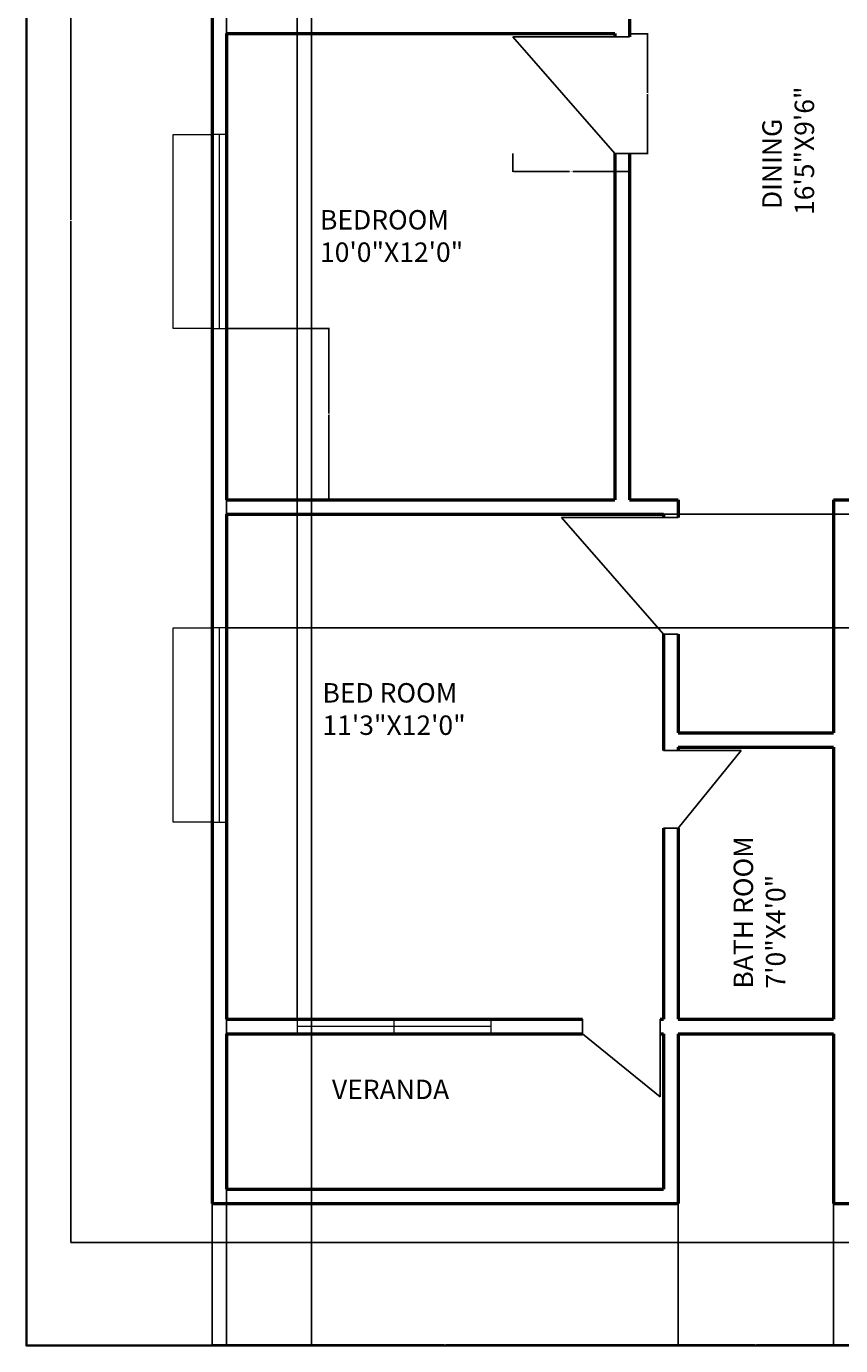
# Model space of a CAD drawing. Units: inches. Extents: x 2412 to 3014, y 10657 to 11360.
# Tile 1 of 3: x 2412 to 2664, y 10657 to 11065. Entities that reach past the tile are written whole.
import ezdxf

# ---------------------------------------------------------------- set-up
doc = ezdxf.new("R2010")
doc.units = ezdxf.units.IN
doc.header["$MEASUREMENT"] = 0
for name, color, linetype, lineweight in [('A-ANNO-DIMS', 2, 'Continuous', 18), ('A-ANNO-TTLB', 7, 'Continuous', 35), ('A-AREA-IDEN', 7, 'Continuous', 18), ('A-DOOR', 22, 'Continuous', 25), ('A-GLAZ', 160, 'Continuous', 18), ('A-WALL', 142, 'Continuous', 50)]:
    doc.layers.add(name, color=color, linetype=linetype, lineweight=lineweight)
doc.styles.get("Standard").update_dxf_attribs({"font": 'arial.ttf'})
doc.dimstyles.get("Standard").update_dxf_attribs({"dimtxt": 0.18, "dimasz": 0.18, "dimexe": 0.18, "dimexo": 0.0625, "dimgap": 0.09, "dimtad": 0, "dimtih": 1, "dimtoh": 1, "dimdec": 4, "dimzin": 0, "dimdsep": 46, "dimtxsty": 'Standard', "dimcen": 0.09, "dimadec": 0, "dimazin": 0, "dimtfac": 1, "dimtdec": 4, "dimtofl": 0, "dimtmove": 0, "dimatfit": 3, "dimfxl": 1, "dimtolj": 1, "dimtzin": 0, "dimarcsym": 0})

# ---------------------------------------------------------------- blocks, each defined once
blk = doc.blocks.new('WIN-60IN-PROJECTING-SILL')
for p, q in [((0, 0), (0, 12)), ((0, 12), (60, 12)), ((60, 12), (60, 0)), ((0, 0), (0, -4.5)), ((60, 0), (0, 0)), ((60, -4.5), (60, 0)), ((60, -2.25), (0, -2.25)), ((0, -4.5), (60, -4.5))]:
    blk.add_line(p, q)
blk = doc.blocks.new('WIN-60IN-DIVIDED')
for p, q in [((0, 0), (0, -4.5)), ((60, 0), (0, 0)), ((30, 0), (30, -4.5)), ((60, -4.5), (60, 0)), ((0, -2.25), (60, -2.25)), ((0, -4.5), (60, -4.5))]:
    blk.add_line(p, q)
blk = doc.blocks.new('DOOR-24IN-DIAGONAL')
for p, q in [((0, 24), (-24, 4.5)), ((0, 0), (0, 24)), ((0, 24), (0, 0)), ((-24, 0), (-24, 4.5)), ((1, 0), (0, 0))]:
    blk.add_line(p, q)
blk = doc.blocks.new('DOOR-36IN-DIAGONAL')
for p, q in [((0, 0), (-36, 0)), ((-36, 0), (0, 0)), ((-36, 0), (-4.5, -36)), ((0, 1), (0, 0)), ((0, -36), (-4.5, -36))]:
    blk.add_line(p, q)
blk = doc.blocks.new('*D18')
at = {"layer": 'A-ANNO-DIMS', "color": 0, "lineweight": -2, "transparency": 16777216}
for p, q in [((2598.92, 11062.78), (2604.59, 11062.78)), ((2604.41, 11062.6), (2604.41, 11044.46)), ((2604.41, 11025.96), (2604.41, 11044.1)), ((2598.92, 11025.78), (2604.59, 11025.78))]:
    blk.add_line(p, q, dxfattribs=at)
at = {"layer": 'A-ANNO-DIMS', "color": 0, "transparency": 16777216}
for points in [[(2604.38, 11062.6), (2604.44, 11062.6), (2604.41, 11062.78)], [(2604.38, 11025.96), (2604.44, 11025.96), (2604.41, 11025.78)]]:
    blk.add_solid(points, dxfattribs=at)
at = {"layer": 'Defpoints', "color": 0, "transparency": 16777216}
for p in [(2598.86, 11062.78), (2604.41, 11062.78), (2598.86, 11025.78)]:
    blk.add_point(p, dxfattribs=at)
at = {"layer": 'A-ANNO-DIMS', "color": 0, "transparency": 16777216, "insert": (2604.41, 11044.28), "char_height": 0.18, "attachment_point": 5}
blk.add_mtext('\\A1;D3 37 TYP.', dxfattribs=at)
blk = doc.blocks.new('*D19')
at = {"layer": 'A-ANNO-DIMS', "color": 0, "lineweight": -2, "transparency": 16777216}
for p, q in [((2562.86, 11025.72), (2562.86, 11020.05)), ((2598.86, 11025.72), (2598.86, 11020.05)), ((2563.04, 11020.23), (2580.33, 11020.23)), ((2598.68, 11020.23), (2581.39, 11020.23))]:
    blk.add_line(p, q, dxfattribs=at)
at = {"layer": 'A-ANNO-DIMS', "color": 0, "transparency": 16777216}
for points in [[(2563.04, 11020.26), (2563.04, 11020.2), (2562.86, 11020.23)], [(2598.68, 11020.26), (2598.68, 11020.2), (2598.86, 11020.23)]]:
    blk.add_solid(points, dxfattribs=at)
at = {"layer": 'Defpoints', "color": 0, "transparency": 16777216}
for p in [(2562.86, 11025.78), (2598.86, 11025.78), (2598.86, 11020.23)]:
    blk.add_point(p, dxfattribs=at)
at = {"layer": 'A-ANNO-DIMS', "color": 0, "transparency": 16777216, "insert": (2580.86, 11020.23), "char_height": 0.18, "attachment_point": 5}
blk.add_mtext('\\A1;36 TYP.', dxfattribs=at)
blk = doc.blocks.new('*D23')
at = {"layer": 'A-ANNO-DIMS', "color": 0, "lineweight": -2, "transparency": 16777216}
for p, q in [((2469.8, 11320.78), (2426.08, 11320.78)), ((2426.26, 11320.6), (2426.26, 11005.21)), ((2426.26, 10689.46), (2426.26, 11004.85)), ((2684.42, 10689.28), (2426.08, 10689.28))]:
    blk.add_line(p, q, dxfattribs=at)
at = {"layer": 'A-ANNO-DIMS', "color": 0, "transparency": 16777216}
for points in [[(2426.23, 11320.6), (2426.29, 11320.6), (2426.26, 11320.78)], [(2426.23, 10689.46), (2426.29, 10689.46), (2426.26, 10689.28)]]:
    blk.add_solid(points, dxfattribs=at)
at = {"layer": 'Defpoints', "color": 0, "transparency": 16777216}
for p in [(2426.26, 11320.78), (2469.86, 11320.78), (2684.48, 10689.28)]:
    blk.add_point(p, dxfattribs=at)
at = {"layer": 'A-ANNO-DIMS', "color": 0, "transparency": 16777216, "insert": (2426.26, 11005.03), "char_height": 0.18, "attachment_point": 5}
blk.add_mtext('\\A1;631.5', dxfattribs=at)
blk = doc.blocks.new('*D24')
at = {"layer": 'A-ANNO-DIMS', "color": 0, "lineweight": -2, "transparency": 16777216}
for p, q in [((2469.86, 10701.22), (2469.86, 10657.5)), ((2613.86, 10701.22), (2613.86, 10657.5)), ((2470.04, 10657.68), (2541.58, 10657.68)), ((2613.68, 10657.68), (2542.14, 10657.68))]:
    blk.add_line(p, q, dxfattribs=at)
at = {"layer": 'A-ANNO-DIMS', "color": 0, "transparency": 16777216}
for points in [[(2470.04, 10657.71), (2470.04, 10657.65), (2469.86, 10657.68)], [(2613.68, 10657.71), (2613.68, 10657.65), (2613.86, 10657.68)]]:
    blk.add_solid(points, dxfattribs=at)
at = {"layer": 'Defpoints', "color": 0, "transparency": 16777216}
for p in [(2469.86, 10701.28), (2613.86, 10701.28), (2613.86, 10657.68)]:
    blk.add_point(p, dxfattribs=at)
at = {"layer": 'A-ANNO-DIMS', "color": 0, "transparency": 16777216, "insert": (2541.86, 10657.68), "char_height": 0.18, "attachment_point": 5}
blk.add_mtext('\\A1;144', dxfattribs=at)
blk = doc.blocks.new('*D25')
at = {"layer": 'A-ANNO-DIMS', "color": 0, "lineweight": -2, "transparency": 16777216}
for p, q in [((2613.86, 10701.22), (2613.86, 10657.5)), ((2661.86, 10701.22), (2661.86, 10657.5)), ((2614.04, 10657.68), (2637.64, 10657.68)), ((2661.68, 10657.68), (2638.08, 10657.68))]:
    blk.add_line(p, q, dxfattribs=at)
at = {"layer": 'A-ANNO-DIMS', "color": 0, "transparency": 16777216}
for points in [[(2614.04, 10657.71), (2614.04, 10657.65), (2613.86, 10657.68)], [(2661.68, 10657.71), (2661.68, 10657.65), (2661.86, 10657.68)]]:
    blk.add_solid(points, dxfattribs=at)
at = {"layer": 'Defpoints', "color": 0, "transparency": 16777216}
for p in [(2613.86, 10701.28), (2661.86, 10701.28), (2661.86, 10657.68)]:
    blk.add_point(p, dxfattribs=at)
at = {"layer": 'A-ANNO-DIMS', "color": 0, "transparency": 16777216, "insert": (2637.86, 10657.68), "char_height": 0.18, "attachment_point": 5}
blk.add_mtext('\\A1;48', dxfattribs=at)
blk = doc.blocks.new('*D26')
at = {"layer": 'A-ANNO-DIMS', "color": 0, "lineweight": -2, "transparency": 16777216}
for p, q in [((2661.86, 10701.22), (2661.86, 10657.5)), ((2768.36, 10701.22), (2768.36, 10657.5)), ((2662.04, 10657.68), (2714.73, 10657.68)), ((2768.18, 10657.68), (2715.5, 10657.68))]:
    blk.add_line(p, q, dxfattribs=at)
at = {"layer": 'A-ANNO-DIMS', "color": 0, "transparency": 16777216}
for points in [[(2662.04, 10657.71), (2662.04, 10657.65), (2661.86, 10657.68)], [(2768.18, 10657.71), (2768.18, 10657.65), (2768.36, 10657.68)]]:
    blk.add_solid(points, dxfattribs=at)
at = {"layer": 'Defpoints', "color": 0, "transparency": 16777216}
for p in [(2661.86, 10701.28), (2768.36, 10701.28), (2768.36, 10657.68)]:
    blk.add_point(p, dxfattribs=at)
at = {"layer": 'A-ANNO-DIMS', "color": 0, "transparency": 16777216, "insert": (2715.11, 10657.68), "char_height": 0.18, "attachment_point": 5}
blk.add_mtext('\\A1;106.5', dxfattribs=at)
blk = doc.blocks.new('*D40')
at = {"layer": 'A-ANNO-DIMS', "color": 0, "lineweight": -2, "transparency": 16777216}
for p, q in [((2474.36, 11263.72), (2474.36, 10657.5)), ((2500.62, 11263.72), (2500.62, 10657.5)), ((2474.54, 10657.68), (2487.1, 10657.68)), ((2500.44, 10657.68), (2487.89, 10657.68))]:
    blk.add_line(p, q, dxfattribs=at)
at = {"layer": 'A-ANNO-DIMS', "color": 0, "transparency": 16777216}
for points in [[(2474.54, 10657.71), (2474.54, 10657.65), (2474.36, 10657.68)], [(2500.44, 10657.71), (2500.44, 10657.65), (2500.62, 10657.68)]]:
    blk.add_solid(points, dxfattribs=at)
at = {"layer": 'Defpoints', "color": 0, "transparency": 16777216}
for p in [(2474.36, 11263.78), (2500.62, 11263.78), (2500.62, 10657.68)]:
    blk.add_point(p, dxfattribs=at)
at = {"layer": 'A-ANNO-DIMS', "color": 0, "transparency": 16777216, "insert": (2487.49, 10657.68), "char_height": 0.18, "attachment_point": 5}
blk.add_mtext('\\A1;26.26', dxfattribs=at)
blk = doc.blocks.new('*D42')
at = {"layer": 'A-ANNO-DIMS', "color": 0, "lineweight": -2, "transparency": 16777216}
for p, q in [((2474.36, 10758.34), (2474.36, 11352.57)), ((2474.54, 11352.39), (2484.85, 11352.39)), ((2495.94, 11352.39), (2485.64, 11352.39)), ((2496.12, 10758.34), (2496.12, 11352.57))]:
    blk.add_line(p, q, dxfattribs=at)
at = {"layer": 'A-ANNO-DIMS', "color": 0, "transparency": 16777216}
for points in [[(2474.54, 11352.42), (2474.54, 11352.36), (2474.36, 11352.39)], [(2495.94, 11352.42), (2495.94, 11352.36), (2496.12, 11352.39)]]:
    blk.add_solid(points, dxfattribs=at)
at = {"layer": 'Defpoints', "color": 0, "transparency": 16777216}
for p in [(2496.12, 11352.39), (2474.36, 10758.28), (2496.12, 10758.28)]:
    blk.add_point(p, dxfattribs=at)
at = {"layer": 'A-ANNO-DIMS', "color": 0, "transparency": 16777216, "insert": (2485.24, 11352.39), "char_height": 0.18, "attachment_point": 5}
blk.add_mtext('\\A1;21.76', dxfattribs=at)
blk = doc.blocks.new('*D45')
at = {"layer": 'A-ANNO-DIMS', "color": 0, "lineweight": -2, "transparency": 16777216}
for p, q in [((2474.42, 10971.64), (2506.15, 10971.64)), ((2505.97, 10971.46), (2505.97, 10945.39)), ((2505.97, 10918.96), (2505.97, 10945.03)), ((2474.42, 10918.78), (2506.15, 10918.78))]:
    blk.add_line(p, q, dxfattribs=at)
at = {"layer": 'A-ANNO-DIMS', "color": 0, "transparency": 16777216}
for points in [[(2505.94, 10971.46), (2506, 10971.46), (2505.97, 10971.64)], [(2505.94, 10918.96), (2506, 10918.96), (2505.97, 10918.78)]]:
    blk.add_solid(points, dxfattribs=at)
at = {"layer": 'Defpoints', "color": 0, "transparency": 16777216}
for p in [(2474.36, 10971.64), (2474.36, 10918.78), (2505.97, 10918.78)]:
    blk.add_point(p, dxfattribs=at)
at = {"layer": 'A-ANNO-DIMS', "color": 0, "transparency": 16777216, "insert": (2505.97, 10945.21), "char_height": 0.18, "attachment_point": 5}
blk.add_mtext('\\A1;52.86', dxfattribs=at)
blk = doc.blocks.new('*D46')
at = {"layer": 'A-ANNO-DIMS', "color": 0, "lineweight": -2, "transparency": 16777216}
for p, q in [((2474.42, 10914.28), (3004.15, 10914.28)), ((3003.97, 10914.1), (3003.97, 10896.9)), ((3003.97, 10879.33), (3003.97, 10896.53)), ((2474.42, 10879.15), (3004.15, 10879.15))]:
    blk.add_line(p, q, dxfattribs=at)
at = {"layer": 'A-ANNO-DIMS', "color": 0, "transparency": 16777216}
for points in [[(3003.94, 10914.1), (3004, 10914.1), (3003.97, 10914.28)], [(3003.94, 10879.33), (3004, 10879.33), (3003.97, 10879.15)]]:
    blk.add_solid(points, dxfattribs=at)
at = {"layer": 'Defpoints', "color": 0, "transparency": 16777216}
for p in [(2474.36, 10914.28), (3003.97, 10914.28), (2474.36, 10879.15)]:
    blk.add_point(p, dxfattribs=at)
at = {"layer": 'A-ANNO-DIMS', "color": 0, "transparency": 16777216, "insert": (3003.97, 10896.71), "char_height": 0.18, "attachment_point": 5}
blk.add_mtext('\\A1;35.13', dxfattribs=at)

msp = doc.modelspace()

# ---------------------------------------------------------------- linework, layer by layer
at = {"layer": 'A-ANNO-TTLB'}
msp.add_lwpolyline([(2412.4885, 11360.4742), (3014.2671, 11360.4742), (3014.2671, 10657.3977), (2412.4885, 10657.3977)], close=True, dxfattribs=at)
at = {"layer": 'A-WALL'}
for p, q in [((2469.8613, 11320.7803), (2469.8613, 10701.2803)), ((2598.8613, 11067.2803), (2598.8613, 11061.7803)), ((2474.3613, 11062.7803), (2594.3613, 11062.7803)), ((2474.3613, 11062.7803), (2474.3613, 10918.7803)), ((2594.3613, 11062.7803), (2594.3613, 11061.7803)), ((2594.3613, 11025.7803), (2594.3613, 10918.7803)), ((2598.8613, 11025.7803), (2598.8613, 10918.7803)), ((2474.3613, 10918.7803), (2594.3613, 10918.7803)), ((2598.8613, 10918.7803), (2613.8613, 10918.7803)), ((2613.8613, 10918.7803), (2613.8613, 10913.2803)), ((2661.8613, 10918.7803), (2661.8613, 10846.7803)), ((2661.8613, 10918.7803), (2675.8613, 10918.7803)), ((2474.3613, 10914.2803), (2609.3613, 10914.2803)), ((2474.3613, 10914.2803), (2474.3613, 10758.2803)), ((2609.3613, 10914.2803), (2609.3613, 10913.2803)), ((2609.3613, 10877.2803), (2609.3613, 10841.2803)), ((2613.8613, 10877.2803), (2613.8613, 10846.7803)), ((2613.8613, 10846.7803), (2661.8613, 10846.7803)), ((2613.8613, 10842.2803), (2661.8613, 10842.2803)), ((2613.8613, 10842.2803), (2613.8613, 10841.2803)), ((2661.8613, 10842.2803), (2661.8613, 10758.2803)), ((2609.3613, 10817.2803), (2609.3613, 10758.2803)), ((2613.8613, 10817.2803), (2613.8613, 10758.2803)), ((2474.3613, 10758.2803), (2584.3613, 10758.2803)), ((2608.3613, 10758.2803), (2609.3613, 10758.2803)), ((2613.8613, 10758.2803), (2661.8613, 10758.2803)), ((2474.3613, 10753.7803), (2584.3613, 10753.7803)), ((2474.3613, 10753.7803), (2474.3613, 10705.7803)), ((2608.3613, 10753.7803), (2609.3613, 10753.7803)), ((2609.3613, 10753.7803), (2609.3613, 10705.7803)), ((2613.8613, 10753.7803), (2661.8613, 10753.7803)), ((2613.8613, 10753.7803), (2613.8613, 10701.2803)), ((2661.8613, 10753.7803), (2661.8613, 10701.2803)), ((2474.3613, 10705.7803), (2609.3613, 10705.7803)), ((2469.8613, 10701.2803), (2613.8613, 10701.2803)), ((2661.8613, 10701.2803), (2768.3613, 10701.2803))]:
    msp.add_line(p, q, dxfattribs=at)

# ---------------------------------------------------------------- block references
at = {"layer": 'A-DOOR'}
for p in [(2598.8613, 11061.7803), (2613.8613, 10913.2803)]:
    msp.add_blockref('DOOR-36IN-DIAGONAL', p, dxfattribs=at)
at = {"layer": 'A-DOOR', "extrusion": (0, 0, -1), "zscale": -1}
for p, rotation in [((-2609.3613, 10841.2803), 89.99999999998668), ((-2608.3613, 10758.2803), 180)]:
    msp.add_blockref('DOOR-24IN-DIAGONAL', p, dxfattribs=dict(at, rotation=rotation))
at = {"layer": 'A-GLAZ'}
for name, p, rotation in [('WIN-60IN-PROJECTING-SILL', (2469.8613, 10971.6386), 90.00000000001131), ('WIN-60IN-PROJECTING-SILL', (2469.8613, 10819.149), 90.00000000001344), ('WIN-60IN-DIVIDED', (2556.1196, 10753.7803), 180)]:
    msp.add_blockref(name, p, dxfattribs=dict(at, rotation=rotation))

# ---------------------------------------------------------------- texts
at = {"layer": 'A-AREA-IDEN', "char_height": 6, "attachment_point": 1, "rotation": 90}
for s, width, insert in [(' DINING\\P16\'5"X9\'6"', 72.937811, (2639.9154, 11006.7462)), ('BATH ROOM\\P7\'0"X4\'0"', 111.272779, (2631.056, 10767.7222))]:
    msp.add_mtext_dynamic_manual_height_columns(s, width=width, gutter_width=30, heights=[0], dxfattribs=dict(at, insert=insert))
at = {"layer": 'A-AREA-IDEN', "char_height": 6, "attachment_point": 1}
for s, width, heights, insert in [('BEDROOM\\P10\'0"X12\'0"', 65.951062, [0], (2503.2287, 11008.2657)), ('BED ROOM\\P11\'3"X12\'0"', 65.606634, [0], (2503.9846, 10862.1068)), ('VERANDA', 60.155979, [6], (2506.9207, 10739.5657))]:
    msp.add_mtext_dynamic_manual_height_columns(s, width=width, gutter_width=30, heights=heights, dxfattribs=dict(at, insert=insert))

# ---------------------------------------------------------------- dimensions: what is measured, and where the dimension line sits
at = {"layer": 'A-ANNO-DIMS'}
for base, p1, p2, override, picture, middle in [((2496.1196, 11352.3853), (2474.3613, 10758.2803), (2496.1196, 10758.2803), {"dimdec": 2, "dimlfac": 1, "dimrnd": 0, "dimzin": 0, "dimdsep": 46, "dimlunit": 2}, '*D42', (2485.2404, 11352.3853)), ((2500.6214, 10657.6753), (2474.3613, 11263.7803), (2500.6214, 11263.7803), {"dimdec": 2, "dimlfac": 1, "dimrnd": 0, "dimzin": 0, "dimdsep": 46, "dimlunit": 2}, '*D40', (2487.4914, 10657.6753)), ((2613.8613, 10657.6753), (2469.8613, 10701.2803), (2613.8613, 10701.2803), {"dimdec": 0, "dimlfac": 1, "dimrnd": 0, "dimzin": 0, "dimdsep": 46, "dimlunit": 2}, '*D24', (2541.8613, 10657.6753)), ((2661.8613, 10657.6753), (2613.8613, 10701.2803), (2661.8613, 10701.2803), {"dimdec": 0, "dimlfac": 1, "dimrnd": 0, "dimzin": 0, "dimdsep": 46, "dimlunit": 2}, '*D25', (2637.8613, 10657.6753)), ((2768.3613, 10657.6753), (2661.8613, 10701.2803), (2768.3613, 10701.2803), {"dimdec": 1, "dimlfac": 1, "dimrnd": 0, "dimzin": 0, "dimdsep": 46, "dimlunit": 2}, '*D26', (2715.1113, 10657.6753))]:
    dim = msp.add_linear_dim(base=base, p1=p1, p2=p2, dimstyle='Standard', override=override, dxfattribs=at)
    dim.commit()
    dim.dimension.update_dxf_attribs({"geometry": picture, "text_midpoint": middle})
for base, p1, p2, angle, override, picture, middle in [((2426.2563, 11320.7803), (2684.4775, 10689.2803), (2469.8613, 11320.7803), 90, {"dimdec": 1, "dimlfac": 1, "dimrnd": 0, "dimzin": 0, "dimdsep": 46, "dimlunit": 2}, '*D23', (2426.2563, 11005.0303)), ((2505.9663, 10918.7803), (2474.3613, 10971.6386), (2474.3613, 10918.7803), 270, {"dimdec": 2, "dimlfac": 1, "dimrnd": 0, "dimzin": 0, "dimdsep": 46, "dimlunit": 2}, '*D45', (2505.9663, 10945.2095)), ((3003.9663, 10914.2803), (2474.3613, 10879.149), (2474.3613, 10914.2803), 90, {"dimdec": 2, "dimlfac": 1, "dimrnd": 0, "dimzin": 0, "dimdsep": 46, "dimlunit": 2}, '*D46', (3003.9663, 10896.7146))]:
    dim = msp.add_linear_dim(base=base, p1=p1, p2=p2, angle=angle, dimstyle='Standard', override=override, dxfattribs=at)
    dim.commit()
    dim.dimension.update_dxf_attribs({"geometry": picture, "text_midpoint": middle})
dim = msp.add_linear_dim(base=(2604.4113, 11062.7803), p1=(2598.8613, 11025.7803), p2=(2598.8613, 11062.7803), angle=90, text='D3 <> TYP.', dimstyle='Standard', override={"dimdec": 0, "dimlfac": 1, "dimrnd": 0, "dimzin": 0, "dimdsep": 46, "dimlunit": 2}, dxfattribs=at)
dim.commit()
dim.dimension.update_dxf_attribs({"geometry": '*D18', "text_midpoint": (2604.4113, 11044.2803)})
dim = msp.add_linear_dim(base=(2598.8613, 11020.2303), p1=(2562.8613, 11025.7803), p2=(2598.8613, 11025.7803), text='<> TYP.', dimstyle='Standard', override={"dimdec": 0, "dimlfac": 1, "dimrnd": 0, "dimzin": 0, "dimdsep": 46, "dimlunit": 2}, dxfattribs=at)
dim.commit()
dim.dimension.update_dxf_attribs({"geometry": '*D19', "text_midpoint": (2580.8613, 11020.2303)})

doc.saveas('drawing.dxf')
